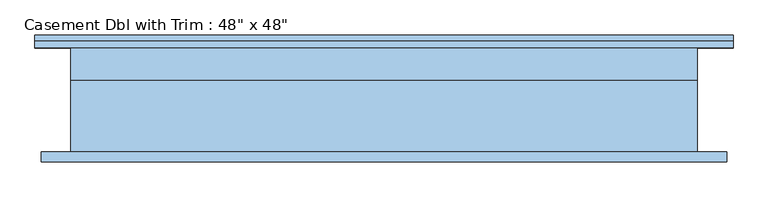
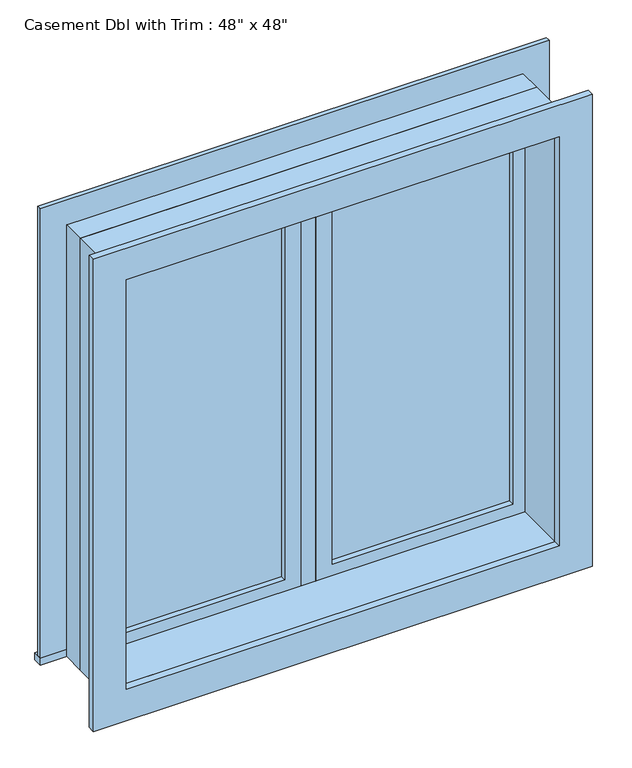
"""IFC4 building model written with IfcOpenShell, lengths in millimetres: window geometry."""

from ifc_helpers import new_model, si_unit, frame, origin, place, context, project, spatial, polyline, outline, extrude, source, transform, mapped, element, save


def window_0862ab64(model_context):
    return source(origin(), model_context, "Body", "SweptSolid", [
        extrude(outline(polyline([(63.5, 85.725), (546.1, 85.725), (546.1, 73.025), (63.5, 73.025), (63.5, 85.725)])), frame((0.0, 0.0, 977.9), z_axis=(0.0, 0.0, 1.0), x_axis=(1.0, 0.0, 0.0)), (0.0, 0.0, 1.0), 1092.2),
        extrude(outline(polyline([(2114.55, 19.05), (933.45, 19.05), (933.45, 590.55), (2114.55, 590.55), (2114.55, 19.05)]), holes=[polyline([(2070.1, 63.5), (2070.1, 546.1), (977.9, 546.1), (977.9, 63.5), (2070.1, 63.5)])]), frame((0.0, 57.15, 0.0), z_axis=(0.0, 1.0, 0.0), x_axis=(0.0, 0.0, 1.0)), (0.0, 0.0, 1.0), 44.45),
        extrude(outline(polyline([(19.05, 57.15), (-19.05, 57.15), (-19.05, 120.65), (19.05, 120.65), (19.05, 57.15)])), frame((0.0, 0.0, 933.45), z_axis=(0.0, 0.0, 1.0), x_axis=(1.0, 0.0, 0.0)), (0.0, 0.0, 1.0), 1181.1),
        extrude(outline(polyline([(-679.45, 146.05), (679.45, 146.05), (679.45, 120.65), (-679.45, 120.65), (-679.45, 146.05)])), frame((0.0, 0.0, 914.4), z_axis=(0.0, 0.0, 1.0), x_axis=(1.0, 0.0, 0.0)), (0.0, 0.0, 1.0), 19.05),
        extrude(outline(polyline([(2114.55, -590.55), (2114.55, 590.55), (933.45, 590.55), (933.45, 679.45), (2203.45, 679.45), (2203.45, -679.45), (933.45, -679.45), (933.45, -590.55), (2114.55, -590.55)])), frame((0.0, 120.65, 0.0), z_axis=(0.0, 1.0, 0.0), x_axis=(0.0, 0.0, 1.0)), (0.0, 0.0, 1.0), 12.7),
        extrude(outline(polyline([(2190.75, 666.75), (2190.75, -666.75), (857.25, -666.75), (857.25, 666.75), (2190.75, 666.75)]), holes=[polyline([(2101.85, 577.85), (946.15, 577.85), (946.15, -577.85), (2101.85, -577.85), (2101.85, 577.85)])]), frame((0.0, -101.6, 0.0), z_axis=(0.0, 1.0, 0.0), x_axis=(0.0, 0.0, 1.0)), (0.0, 0.0, 1.0), 19.05),
        extrude(outline(polyline([(-63.5, 73.025), (-546.1, 73.025), (-546.1, 85.725), (-63.5, 85.725), (-63.5, 73.025)])), frame((0.0, 0.0, 977.9), z_axis=(0.0, 0.0, 1.0), x_axis=(1.0, 0.0, 0.0)), (0.0, 0.0, 1.0), 1092.2),
        extrude(outline(polyline([(2114.55, -590.55), (933.45, -590.55), (933.45, -19.05), (2114.55, -19.05), (2114.55, -590.55)]), holes=[polyline([(2070.1, -546.1), (2070.1, -63.5), (977.9, -63.5), (977.9, -546.1), (2070.1, -546.1)])]), frame((0.0, 57.15, 0.0), z_axis=(0.0, 1.0, 0.0), x_axis=(0.0, 0.0, 1.0)), (0.0, 0.0, 1.0), 44.45),
        extrude(outline(polyline([(2133.6, -609.6), (914.4, -609.6), (914.4, 609.6), (2133.6, 609.6), (2133.6, -609.6)]), holes=[polyline([(2101.85, -577.85), (2101.85, 577.85), (946.15, 577.85), (946.15, -577.85), (2101.85, -577.85)])]), frame((0.0, -82.55, 0.0), z_axis=(0.0, 1.0, 0.0), x_axis=(0.0, 0.0, 1.0)), (0.0, 0.0, 1.0), 139.7),
        extrude(outline(polyline([(2133.6, 609.6), (2133.6, -609.6), (914.4, -609.6), (914.4, 609.6), (2133.6, 609.6)]), holes=[polyline([(2114.55, 590.55), (933.45, 590.55), (933.45, -590.55), (2114.55, -590.55), (2114.55, 590.55)])]), frame((0.0, 57.15, 0.0), z_axis=(0.0, 1.0, 0.0), x_axis=(0.0, 0.0, 1.0)), (0.0, 0.0, 1.0), 63.5),
    ])


if __name__ == "__main__":
    model = new_model("IFC4")
    model_context = context("Model", 3, world=origin())
    ifc_project = project(units=[si_unit("LENGTHUNIT", "METRE", prefix="MILLI")], contexts=[model_context])
    site = spatial("IfcSite", under=ifc_project)
    building = spatial("IfcBuilding", under=site)
    placement = place(None, origin())
    window_shape = window_0862ab64(model_context)
    element("IfcWindow", 1, ObjectType="Casement Dbl with Trim : 48\" x 48\"", at=placement, inside=building, context=model_context, shape_type="MappedRepresentation", body=[
        mapped(window_shape, transform((0.0, 0.0, 0.0), x_axis=(1.0, 0.0, 0.0), y_axis=(0.0, 1.0, 0.0), z_axis=(0.0, 0.0, 1.0))),
    ])
    save(model, "model.ifc")

# Revit data of these elements
# Type "Casement Dbl with Trim : 48\" x 48\""
#   Type Mark = "23"
#   Construction Type Id = "GSP4R"
#   Assembly Code = "B2020100"
#   Analytic Construction = "1/8 in Pilkington single glazing"
#   Visual Light Transmittance = 0.9
#   Solar Heat Gain Coefficient = 0.78
#   Heat Transfer Coefficient (U) = 0.6496 BTU/(h·ft²·°F)
#   Height = 4' - 0"
#   Default Sill Height = 3' - 0"
#   Trim Projection - Ext. = 0' - 0 1/2"
#   Trim Projection - Int. = 0' - 0 3/4"
#   Trim Width - Exterior = 0' - 3 1/2"
#   Trim Width - Interior = 0' - 3 1/2"
#   Width = 4' - 0"
#   Window Inset = 0' - 0 3/4"
#   Define Thermal Properties by = 1
#   Glass Pane Material = Glass
#   Sash Material = Sash
#   Trim Exterior Material = Trim
#   Trim Interior Material = Trim
#   Wall Closure = (empty or 0)
# Element 1 (IfcWindow, "Casement Dbl with Trim : 48\" x 48\"")
#   Materials on its faces: "Sash", "Trim", "Glass"
# Materials
#   "Glass": class "Glass", colour RGB 0 128 192, transparency 0.75, Description = "Soda Lime Glass", Cost = 0
#   "Sash": class "Wood", colour RGB 224 178 126, transparency 0
#   "Trim": class "Wood", colour RGB 224 178 126, transparency 0
